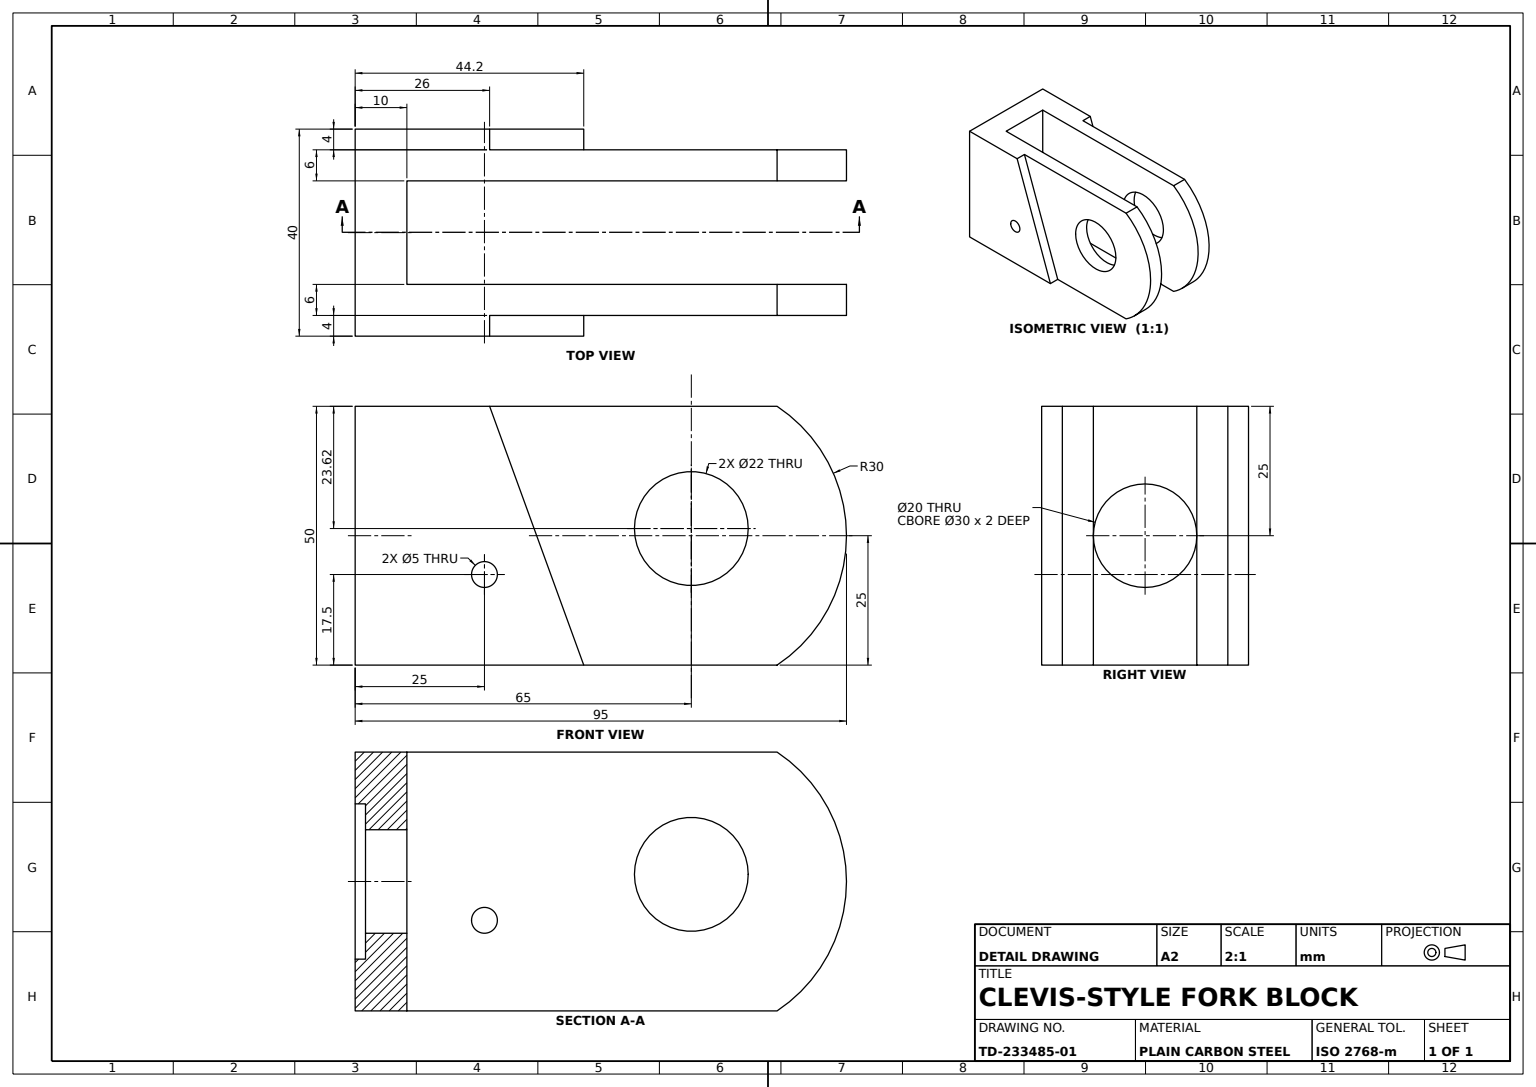
SolidWorks part; units mm, degrees
material "Plain Carbon Steel"
ref_plane "Front Plane" through (0, 0, 0) normal (0, 0, 1) x (1, 0, 0)
ref_plane "Top Plane" through (0, 0, 0) normal (0, 1, 0) x (1, 0, 0)
ref_plane "Right Plane" through (0, 0, 0) normal (1, 0, 0) x (0, 0, -1)
sketch "Side Plate Sketch" plane through (0, 0, 0) normal (0, 0, 1) x (1, 0, 0)
  line L0 (0, 0) -> (0, -50)
  line L1 (0, -50) -> (61.5789, -50)
  line L2 (0, 0) -> (61.5789, 0)
  line L4 (61.5789, 0) -> (77.2893, 0)
  line L5 (77.2893, 0) -> (81.5831, 0)
  line L6 (77.2893, -50) -> (61.5789, -50)
  line L7 (77.2893, -50) -> (81.5831, -50)
  arc A1 (81.5831, -50) -> (81.5831, 0) centre (65, -25) ccw
  point P10 (95, -25)
  dimension "D1" = 50
  dimension "D2" = 65
  dimension "D3" = 95
  dimension "D4" = 61.5789
  dimension "D5" = 77.2893
extrude "Side Plate" add sketch "Side Plate Sketch" along normal blind 10
sketch "Mounting Block Sketch" plane through (0, 0, 0) normal (-1, 0, 0) x (0, 0, 1)
  line L0 (10, 0) -> (40, 0)
  line L1 (40, 0) -> (40, -50)
  line L2 (40, -50) -> (10, -50)
  line L3 (10, -50) -> (10, 0)
  line L4 (0, 0) -> (0, -50) construction
  dimension "D1" = 40
extrude "Mounting Block" add sketch "Mounting Block Sketch" against normal blind 10
sketch "Second Plate Sketch" plane through (0, 0, 40) normal (0, 0, 1) x (1, 0, 0)
  line L0 (10, 0) -> (81.5831, 0)
  line L2 (81.5831, -50) -> (10, -50)
  line L3 (10, -50) -> (10, 0)
  arc A1 (81.5831, -50) -> (81.5831, 0) centre (65, -25) ccw
extrude "Second Side Plate" add sketch "Second Plate Sketch" against normal blind 10
sketch "Top Recess Sketch" plane through (0, 0, 40) normal (0, 0, 1) x (1, 0, 0)
  line L0 (0, -50) -> (0, 0) construction
  line L1 (81.5831, 0) -> (0, 0) construction
  line L2 (0, 0) -> (0, -50)
  line L3 (26, 0) -> (44.1968, -50)
  line L4 (26, 0) -> (81.5831, 0)
  line L5 (81.5831, -50) -> (0, -50) construction
  line L7 (81.5831, -50) -> (44.1968, -50)
  arc A1 (81.5831, -50) -> (81.5831, 0) centre (65, -25) ccw
  line M2 (0, -50) -> (81.5831, -50)
  arc M3 (81.5831, -50) -> (81.5831, 0) centre (65, -25) ccw
  line M4 (81.5831, 0) -> (0, 0)
  dimension "D1" = 26
  dimension "D2" = 44.1968
extrude "Top Recess 4mm" cut sketch "Top Recess Sketch" against normal blind 4 contours L3 M4 M2 M3
sketch "Hole Axis Sketch" plane through (0, 0, 0) normal (0, 0, -1) x (-1, 0, 0)
  line L0 (0, 0) -> (0, -50)
sketch "Side Recess Sketch" plane through (0, 0, 0) normal (0, 0, -1) x (-1, 0, 0)
  line L1 (0, -50) -> (-81.5831, -50) construction
  line L4 (-81.5831, 0) -> (0, 0) construction
  line L5 (-26, 0) -> (-44.2, -50)
  line L6 (-26, 0) -> (-81.5831, 0)
  line L7 (0, 0) -> (0, -50) construction
  line L8 (-81.5831, -50) -> (-44.2, -50)
  arc A0 (-81.5831, 0) -> (-81.5831, -50) centre (-65, -25) ccw
  dimension "D1" = 26
  dimension "D2" = 44.2
extrude "Side Recess 4mm" cut sketch "Side Recess Sketch" against normal blind 4
sketch "Cross Hole Sketch" plane through (0, 0, 36) normal (0, 0, 1) x (1, 0, 0)
  line L0 (0, 0) -> (0, -50) construction
  line L1 (81.5831, 0) -> (26, 0) construction
  circle A0 centre (65, -23.6192) radius 11
  dimension "D1" = 65
  dimension "D2" = 22
  dimension "D3" = 23.6192
extrude "Cross Hole" cut sketch "Cross Hole Sketch" against normal blind 40
sketch "Spot Face Sketch" plane through (0, 0, 0) normal (-1, 0, 0) x (0, 0, 1)
  line L0 (0, 0) -> (0, -50) construction
  line L1 (40, -50) -> (0, -50) construction
  circle A0 centre (20, -25) radius 15
  dimension "D1" = 30
  dimension "D2" = 20
  dimension "D3" = 25
extrude "Spot Face 2mm" cut sketch "Spot Face Sketch" against normal blind 2
sketch "Small Hole Sketch" plane through (2, 0, 0) normal (-1, 0, 0) x (0, 0, 1)
  circle A0 centre (20, -25) radius 10
  dimension "D1" = 20
extrude "Small Hole 15mm Deep" cut sketch "Small Hole Sketch" against normal blind 15
sketch "Pin Hole Sketch" plane through (0, 0, 40) normal (0, 0, 1) x (1, 0, 0)
  line L0 (44.1968, -50) -> (0, -50) construction
  line L1 (0, 0) -> (0, -50) construction
  circle A0 centre (25, -32.5) radius 2.5
  dimension "D1" = 17.5
  dimension "D3" = 5
  dimension "D2" = 25
extrude "Pin Hole" cut sketch "Pin Hole Sketch" against normal blind 40
